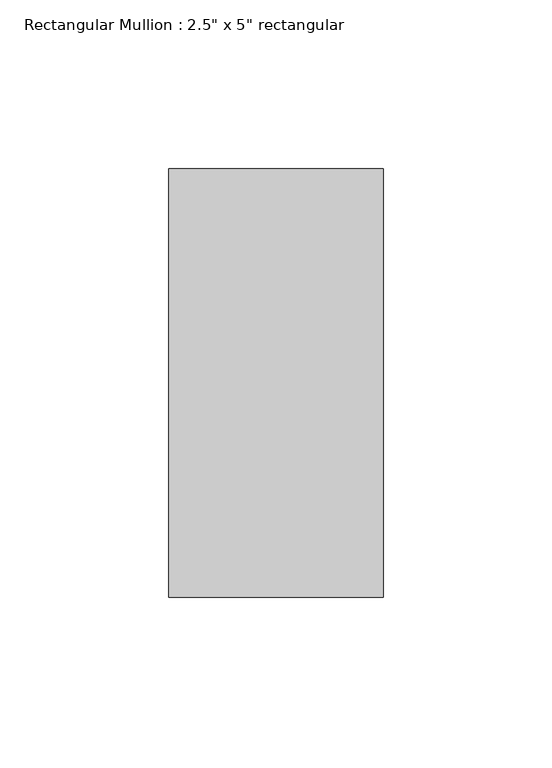
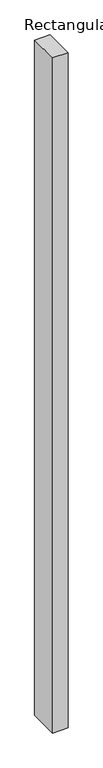
"""IFC4 building model written with IfcOpenShell, lengths in millimetres: member geometry."""

from ifc_helpers import new_model, si_unit, frame, origin, place, context, project, spatial, polyline, outline, extrude, source, transform, mapped, element, save


def member_d457d5cf(model_context):
    return source(origin(), model_context, "Body", "SweptSolid", [
        extrude(outline(polyline([(0.0, 63.5), (0.0, -63.5), (-63.5, -63.5), (-63.5, 63.5), (0.0, 63.5)])), frame((0.0, 0.0, -2921.0), z_axis=(0.0, 0.0, 1.0), x_axis=(1.0, 0.0, 0.0)), (0.0, 0.0, 1.0), 2921.0),
    ])


if __name__ == "__main__":
    model = new_model("IFC4")
    model_context = context("Model", 3, world=origin())
    ifc_project = project(units=[si_unit("LENGTHUNIT", "METRE", prefix="MILLI")], contexts=[model_context])
    site = spatial("IfcSite", under=ifc_project)
    building = spatial("IfcBuilding", under=site)
    placement = place(None, origin())
    member_shape = member_d457d5cf(model_context)
    element("IfcMember", 1, ObjectType="Rectangular Mullion : 2.5\" x 5\" rectangular", at=placement, inside=building, context=model_context, shape_type="MappedRepresentation", body=[
        mapped(member_shape, transform((0.0, 0.0, 0.0), x_axis=(1.0, 0.0, 0.0), y_axis=(0.0, 1.0, 0.0), z_axis=(0.0, 0.0, 1.0))),
    ])
    save(model, "model.ifc")

# Revit data of these elements
# Type "Rectangular Mullion : 2.5\" x 5\" rectangular"
#   built-in parameter 1007304 = 0.416667 (stored number, unit not read)
#   built-in parameter 1007301 = 0.104167 (stored number, unit not read)
#   built-in parameter 1007300 = 0.104167 (stored number, unit not read)
# Element 1 (IfcMember, "Rectangular Mullion : 2.5\" x 5\" rectangular")
#   Materials on its faces: "Aluminum"
# Materials
#   "Aluminum": class "Metal", colour RGB 247 247 247, transparency 0, Description = "Aluminum 6061", Cost = 0
